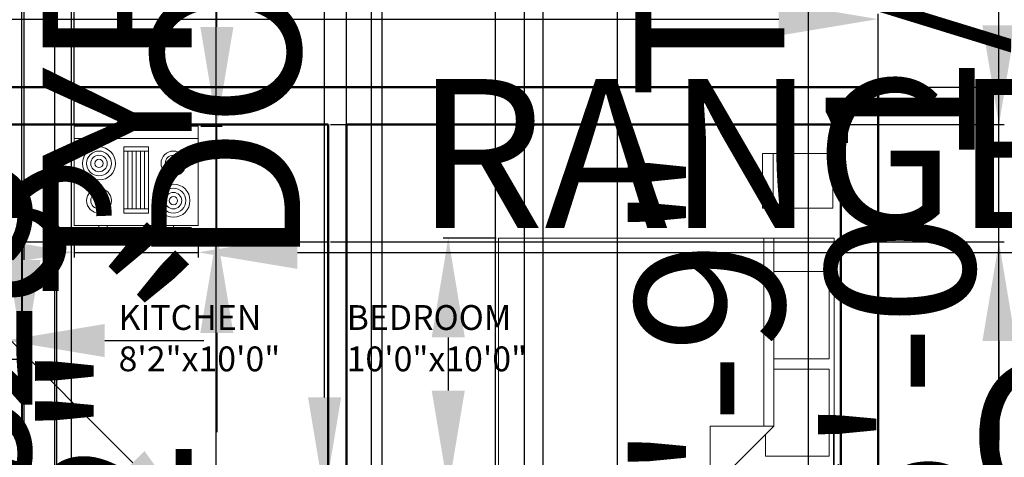
# Model space of a CAD drawing. Units: inches. Extents: x 1102 to 2414, y 295 to 1561.
# Tile 8 of 11: x 1610 to 1848, y 1027 to 1133. Entities that reach past the tile are written whole.
import ezdxf

# ---------------------------------------------------------------- set-up
doc = ezdxf.new("R2010")
doc.units = ezdxf.units.IN
for name, color, linetype, lineweight in [('A-ANNO-DIMS', 2, 'Continuous', 18), ('A-AREA-IDEN', 7, 'Continuous', 25), ('A-EQPM', 9, 'Continuous', 18), ('A-FLOR-CASE', 8, 'Continuous', 25), ('A-FURN', 8, 'Continuous', 18), ('A-WALL', 7, 'Continuous', 50)]:
    doc.layers.add(name, color=color, linetype=linetype, lineweight=lineweight)
doc.styles.get("Standard").update_dxf_attribs({"font": 'arial.ttf'})
doc.dimstyles.new('ISO-25', dxfattribs={"dimtxt": 36, "dimasz": 24, "dimexe": 1.25, "dimexo": 0.625, "dimtad": 1, "dimlunit": 4, "dimtxsty": 'Standard', "dimcen": 2.5, "dimadec": 0, "dimazin": 0, "dimtfac": 1, "dimtmove": 0, "dimatfit": 3, "dimfxl": 1, "dimarcsym": 0})

# ---------------------------------------------------------------- blocks, each defined once
blk = doc.blocks.new('*D1')
at = {"layer": 'A-ANNO-DIMS', "color": 0, "lineweight": -2, "transparency": 16777216}
for p, q in [((1577.54, 1117.38), (1577.54, 1134.48)), ((1817.54, 1117.38), (1817.54, 1134.48)), ((1601.54, 1133.23), (1793.54, 1133.23))]:
    blk.add_line(p, q, dxfattribs=at)
at = {"layer": 'A-ANNO-DIMS', "color": 0, "transparency": 16777216}
for points in [[(1601.54, 1137.23), (1601.54, 1129.23), (1577.54, 1133.23)], [(1793.54, 1137.23), (1793.54, 1129.23), (1817.54, 1133.23)]]:
    blk.add_solid(points, dxfattribs=at)
at = {"layer": 'Defpoints', "color": 0, "transparency": 16777216}
for p in [(1817.54, 1133.23), (1577.54, 1116.76), (1817.54, 1116.76)]:
    blk.add_point(p, dxfattribs=at)
at = {"layer": 'A-ANNO-DIMS', "color": 0, "transparency": 16777216, "insert": (1697.54, 1152.24), "char_height": 36, "attachment_point": 5}
blk.add_mtext("20'", dxfattribs=at)
blk = doc.blocks.new('*D3')
at = {"layer": 'A-ANNO-DIMS', "color": 0, "lineweight": -2, "transparency": 16777216}
for p, q in [((1818.17, 1116.76), (1895.42, 1116.76)), ((1894.17, 1092.76), (1894.17, 660.76)), ((1818.17, 636.76), (1895.42, 636.76))]:
    blk.add_line(p, q, dxfattribs=at)
at = {"layer": 'A-ANNO-DIMS', "color": 0, "transparency": 16777216}
for points in [[(1890.17, 1092.76), (1898.17, 1092.76), (1894.17, 1116.76)], [(1890.17, 660.76), (1898.17, 660.76), (1894.17, 636.76)]]:
    blk.add_solid(points, dxfattribs=at)
at = {"layer": 'Defpoints', "color": 0, "transparency": 16777216}
for p in [(1817.54, 1116.76), (1817.54, 636.76), (1894.17, 636.76)]:
    blk.add_point(p, dxfattribs=at)
at = {"layer": 'A-ANNO-DIMS', "color": 0, "transparency": 16777216, "insert": (1875.16, 876.76), "char_height": 36, "attachment_point": 5, "rotation": 90}
blk.add_mtext("40'", dxfattribs=at)
blk = doc.blocks.new('Range-Oven - 30 in top')
for p, q in [((0, -3), (30, -3)), ((12, -6), (18, -6)), ((13, -20), (13, -6)), ((14, -6), (14, -20)), ((15, -20), (15, -6)), ((16, -6), (16, -20)), ((17, -20), (17, -6)), ((18, -20), (12, -20)), ((6, -24), (6, -25)), ((8, -25), (8, -24)), ((22, -25), (22, -24)), ((24, -24), (24, -25))]:
    blk.add_line(p, q)
for points in [[(0, -24), (0, 0), (30, 0), (30, -24)], [(12, -21), (12, -5), (18, -5), (18, -21)], [(2, -26), (2, -25), (28, -25), (28, -26)]]:
    blk.add_lwpolyline(points, close=True)
for centre, radius in [((6, -9), 4), ((6, -9), 3), ((6, -9), 2), ((24, -9), 3), ((24, -9), 2), ((6, -9), 1), ((24, -9), 1), ((24, -18), 4), ((6, -18), 3), ((6, -18), 2), ((24, -18), 3), ((24, -18), 2), ((6, -18), 1), ((24, -18), 1)]:
    blk.add_circle(centre, radius)
blk = doc.blocks.new('Bed - Queen')
for p, q in [((0, -80.00003), (0, 0)), ((0, 0), (59.99999, 0)), ((59.99999, 0), (59.99999, -80.00003)), ((7.99999, -1.2), (28.79998, -1.2)), ((7.99999, -14.4), (7.99999, -1.2)), ((28.79998, -1.2), (28.79998, -14.4)), ((31.19999, -1.2), (51.99999, -1.2)), ((31.19999, -14.4), (31.19999, -1.2)), ((51.99999, -1.2), (51.99999, -16.4)), ((0, -14.4), (44.8, -14.4)), ((59.99999, -29.6), (44.8, -14.4)), ((44.8, -14.4), (44.8, -29.6)), ((51.99999, -16.4), (46.79936, -16.4)), ((44.8, -16.8), (0, -16.8)), ((44.8, -29.6), (59.99999, -29.6)), ((59.99999, -80.00003), (0, -80.00003))]:
    blk.add_line(p, q)
blk = doc.blocks.new('TABLE-BEDSIDE')
for p, q in [((16.99, 13.29), (0, 13.29)), ((0, 13.29), (0, 0)), ((2.56, 0), (2.56, 13.29)), ((16.99, 0), (16.99, 13.29)), ((0, 0), (16.99, 0))]:
    blk.add_line(p, q)
blk = doc.blocks.new('*D23')
at = {"layer": 'A-ANNO-DIMS', "color": 0, "lineweight": -2, "transparency": 16777216}
for p, q in [((1725.8, 1018.76), (1725.8, 1005.96)), ((1806.97, 1018.76), (1806.97, 1005.96)), ((1749.8, 1007.21), (1782.97, 1007.21)), ((1806.97, 1007.21), (2238.05, 1007.21))]:
    blk.add_line(p, q, dxfattribs=at)
at = {"layer": 'A-ANNO-DIMS', "color": 0, "transparency": 16777216}
for points in [[(1749.8, 1011.21), (1749.8, 1003.21), (1725.8, 1007.21)], [(1782.97, 1011.21), (1782.97, 1003.21), (1806.97, 1007.21)]]:
    blk.add_solid(points, dxfattribs=at)
at = {"layer": 'Defpoints', "color": 0, "transparency": 16777216}
for p in [(1725.8, 1019.39), (1806.97, 1019.39), (1806.97, 1007.21)]:
    blk.add_point(p, dxfattribs=at)
at = {"layer": 'A-ANNO-DIMS', "color": 0, "transparency": 16777216, "insert": (2034.51, 1027.55), "char_height": 36, "attachment_point": 5}
blk.add_mtext('QUEEN BED 6\'-9"', dxfattribs=at)
blk = doc.blocks.new('*D24')
at = {"layer": 'A-ANNO-DIMS', "color": 0, "lineweight": -2, "transparency": 16777216}
for p, q in [((1725.17, 1080.27), (1712.37, 1080.27)), ((1713.62, 1056.27), (1713.62, 1043.39)), ((1725.17, 1019.39), (1712.37, 1019.39)), ((1713.62, 1019.39), (1713.62, 898.44))]:
    blk.add_line(p, q, dxfattribs=at)
at = {"layer": 'A-ANNO-DIMS', "color": 0, "transparency": 16777216}
for points in [[(1709.62, 1056.27), (1717.62, 1056.27), (1713.62, 1080.27)], [(1709.62, 1043.39), (1717.62, 1043.39), (1713.62, 1019.39)]]:
    blk.add_solid(points, dxfattribs=at)
at = {"layer": 'Defpoints', "color": 0, "transparency": 16777216}
for p in [(1725.8, 1080.27), (1713.62, 1019.39), (1725.8, 1019.39)]:
    blk.add_point(p, dxfattribs=at)
at = {"layer": 'A-ANNO-DIMS', "color": 0, "transparency": 16777216, "insert": (1694.62, 946.91), "char_height": 36, "attachment_point": 5, "rotation": 90}
blk.add_mtext('5\'-1"', dxfattribs=at)
blk = doc.blocks.new('*D25')
at = {"layer": 'A-ANNO-DIMS', "color": 0, "lineweight": -2, "transparency": 16777216}
for p, q in [((1800.76, 877.69), (1800.76, 1221.61)), ((1796.43, 853.69), (1802.01, 853.69)), ((1800.76, 820.65), (1800.76, 853.69)), ((1796.43, 820.65), (1802.01, 820.65)), ((1800.76, 796.65), (1800.76, 772.65))]:
    blk.add_line(p, q, dxfattribs=at)
at = {"layer": 'A-ANNO-DIMS', "color": 0, "transparency": 16777216}
for points in [[(1796.76, 877.69), (1804.76, 877.69), (1800.76, 853.69)], [(1796.76, 796.65), (1804.76, 796.65), (1800.76, 820.65)]]:
    blk.add_solid(points, dxfattribs=at)
at = {"layer": 'Defpoints', "color": 0, "transparency": 16777216}
for p in [(1795.81, 853.69), (1800.76, 853.69), (1795.81, 820.65)]:
    blk.add_point(p, dxfattribs=at)
at = {"layer": 'A-ANNO-DIMS', "color": 0, "transparency": 16777216, "insert": (1781.53, 1061.65), "char_height": 36, "attachment_point": 5, "rotation": 90}
blk.add_mtext('WC 2\'-9" TYP.', dxfattribs=at)
blk = doc.blocks.new('*D27')
at = {"layer": 'A-ANNO-DIMS', "color": 0, "lineweight": -2, "transparency": 16777216}
for p, q in [((1683.72, 1041.76), (1683.72, 1561.36)), ((1679.17, 1017.76), (1684.97, 1017.76)), ((1683.72, 983.26), (1683.72, 1017.76)), ((1679.17, 983.26), (1684.97, 983.26)), ((1683.72, 959.26), (1683.72, 935.26))]:
    blk.add_line(p, q, dxfattribs=at)
at = {"layer": 'A-ANNO-DIMS', "color": 0, "transparency": 16777216}
for points in [[(1679.72, 1041.76), (1687.72, 1041.76), (1683.72, 1017.76)], [(1679.72, 959.26), (1687.72, 959.26), (1683.72, 983.26)]]:
    blk.add_solid(points, dxfattribs=at)
at = {"layer": 'Defpoints', "color": 0, "transparency": 16777216}
for p in [(1678.54, 1017.76), (1683.72, 1017.76), (1678.54, 983.26)]:
    blk.add_point(p, dxfattribs=at)
at = {"layer": 'A-ANNO-DIMS', "color": 0, "transparency": 16777216, "insert": (1664.47, 1313.56), "char_height": 36, "attachment_point": 5, "rotation": 90}
blk.add_mtext('DOOR 2\'-10 1/2" TYP.', dxfattribs=at)
blk = doc.blocks.new('*D28')
at = {"layer": 'A-ANNO-DIMS', "color": 0, "lineweight": -2, "transparency": 16777216}
for p, q in [((1645.54, 982.63), (1645.54, 976.83)), ((1678.54, 982.63), (1678.54, 976.83)), ((1621.54, 978.08), (1597.54, 978.08)), ((1645.54, 978.08), (1678.54, 978.08)), ((1702.54, 978.08), (1947.85, 978.08))]:
    blk.add_line(p, q, dxfattribs=at)
at = {"layer": 'A-ANNO-DIMS', "color": 0, "transparency": 16777216}
for points in [[(1621.54, 982.08), (1621.54, 974.08), (1645.54, 978.08)], [(1702.54, 982.08), (1702.54, 974.08), (1678.54, 978.08)]]:
    blk.add_solid(points, dxfattribs=at)
at = {"layer": 'Defpoints', "color": 0, "transparency": 16777216}
for p in [(1645.54, 983.26), (1678.54, 983.26), (1678.54, 978.08)]:
    blk.add_point(p, dxfattribs=at)
at = {"layer": 'A-ANNO-DIMS', "color": 0, "transparency": 16777216, "insert": (1837.19, 997.09), "char_height": 36, "attachment_point": 5}
blk.add_mtext('2\'-9" TYP.', dxfattribs=at)
blk = doc.blocks.new('*D29')
at = {"layer": 'A-ANNO-DIMS', "color": 0, "lineweight": -2, "transparency": 16777216}
for p, q in [((1806.82, 1011.76), (1806.82, 1035.76)), ((1803.17, 987.76), (1808.07, 987.76)), ((1806.82, 987.76), (1806.82, 959.26)), ((1803.17, 959.26), (1808.07, 959.26)), ((1806.82, 935.26), (1806.82, 295.33))]:
    blk.add_line(p, q, dxfattribs=at)
at = {"layer": 'A-ANNO-DIMS', "color": 0, "transparency": 16777216}
for points in [[(1802.82, 1011.76), (1810.82, 1011.76), (1806.82, 987.76)], [(1802.82, 935.26), (1810.82, 935.26), (1806.82, 959.26)]]:
    blk.add_solid(points, dxfattribs=at)
at = {"layer": 'Defpoints', "color": 0, "transparency": 16777216}
for p in [(1802.54, 987.76), (1802.54, 959.26), (1806.82, 959.26)]:
    blk.add_point(p, dxfattribs=at)
at = {"layer": 'A-ANNO-DIMS', "color": 0, "transparency": 16777216, "insert": (1787.57, 603.3), "char_height": 36, "attachment_point": 5, "rotation": 90}
blk.add_mtext('BATH DOOR 2\'-4 1/2" TYP.', dxfattribs=at)
blk = doc.blocks.new('*D30')
at = {"layer": 'A-ANNO-DIMS', "color": 0, "lineweight": -2, "transparency": 16777216}
for p, q in [((1775.54, 988.38), (1775.54, 993.28)), ((1802.54, 988.38), (1802.54, 993.28)), ((1751.54, 992.03), (1727.54, 992.03)), ((1775.54, 992.03), (1802.54, 992.03)), ((1826.54, 992.03), (2071.85, 992.03))]:
    blk.add_line(p, q, dxfattribs=at)
at = {"layer": 'A-ANNO-DIMS', "color": 0, "transparency": 16777216}
for points in [[(1751.54, 996.03), (1751.54, 988.03), (1775.54, 992.03)], [(1826.54, 996.03), (1826.54, 988.03), (1802.54, 992.03)]]:
    blk.add_solid(points, dxfattribs=at)
at = {"layer": 'Defpoints', "color": 0, "transparency": 16777216}
for p in [(1802.54, 992.03), (1775.54, 987.76), (1802.54, 987.76)]:
    blk.add_point(p, dxfattribs=at)
at = {"layer": 'A-ANNO-DIMS', "color": 0, "transparency": 16777216, "insert": (1961.19, 1011.05), "char_height": 36, "attachment_point": 5}
blk.add_mtext('2\'-3" TYP.', dxfattribs=at)
blk = doc.blocks.new('*D32')
at = {"layer": 'A-ANNO-DIMS', "color": 0, "lineweight": -2, "transparency": 16777216}
for p, q in [((1657.46, 811.76), (1657.46, 1164.91)), ((1654.49, 787.76), (1658.71, 787.76)), ((1657.46, 765.26), (1657.46, 787.76)), ((1654.49, 765.26), (1658.71, 765.26)), ((1657.46, 741.26), (1657.46, 717.26))]:
    blk.add_line(p, q, dxfattribs=at)
at = {"layer": 'A-ANNO-DIMS', "color": 0, "transparency": 16777216}
for points in [[(1653.46, 811.76), (1661.46, 811.76), (1657.46, 787.76)], [(1653.46, 741.26), (1661.46, 741.26), (1657.46, 765.26)]]:
    blk.add_solid(points, dxfattribs=at)
at = {"layer": 'Defpoints', "color": 0, "transparency": 16777216}
for p in [(1653.86, 787.76), (1657.46, 787.76), (1653.86, 765.26)]:
    blk.add_point(p, dxfattribs=at)
at = {"layer": 'A-ANNO-DIMS', "color": 0, "transparency": 16777216, "insert": (1638.22, 1000.34), "char_height": 36, "attachment_point": 5, "rotation": 90}
blk.add_mtext('1\'-10 1/2" TYP.', dxfattribs=at)
blk = doc.blocks.new('*D33')
at = {"layer": 'A-ANNO-DIMS', "color": 0, "lineweight": -2, "transparency": 16777216}
for p, q in [((1623.16, 1080.7), (1623.16, 1075.57)), ((1653.16, 1080.7), (1653.16, 1075.57)), ((1599.16, 1076.82), (1575.16, 1076.82)), ((1623.16, 1076.82), (1653.16, 1076.82)), ((1677.16, 1076.82), (1989.06, 1076.82))]:
    blk.add_line(p, q, dxfattribs=at)
at = {"layer": 'A-ANNO-DIMS', "color": 0, "transparency": 16777216}
for points in [[(1599.16, 1080.82), (1599.16, 1072.82), (1623.16, 1076.82)], [(1677.16, 1080.82), (1677.16, 1072.82), (1653.16, 1076.82)]]:
    blk.add_solid(points, dxfattribs=at)
at = {"layer": 'Defpoints', "color": 0, "transparency": 16777216}
for p in [(1623.16, 1081.32), (1653.16, 1081.32), (1653.16, 1076.82)]:
    blk.add_point(p, dxfattribs=at)
at = {"layer": 'A-ANNO-DIMS', "color": 0, "transparency": 16777216, "insert": (1845.11, 1096.06), "char_height": 36, "attachment_point": 5}
blk.add_mtext('RANGE 2\'-6"', dxfattribs=at)
blk = doc.blocks.new('*D34')
at = {"layer": 'A-ANNO-DIMS', "color": 0, "lineweight": -2, "transparency": 16777216}
for p, q in [((1657.66, 1131.32), (1657.66, 1252.88)), ((1653.79, 1107.32), (1658.91, 1107.32)), ((1657.66, 1081.32), (1657.66, 1107.32)), ((1653.79, 1081.32), (1658.91, 1081.32)), ((1657.66, 1057.32), (1657.66, 1033.32))]:
    blk.add_line(p, q, dxfattribs=at)
at = {"layer": 'A-ANNO-DIMS', "color": 0, "transparency": 16777216}
for points in [[(1653.66, 1131.32), (1661.66, 1131.32), (1657.66, 1107.32)], [(1653.66, 1057.32), (1661.66, 1057.32), (1657.66, 1081.32)]]:
    blk.add_solid(points, dxfattribs=at)
at = {"layer": 'Defpoints', "color": 0, "transparency": 16777216}
for p in [(1653.16, 1107.32), (1657.66, 1107.32), (1653.16, 1081.32)]:
    blk.add_point(p, dxfattribs=at)
at = {"layer": 'A-ANNO-DIMS', "color": 0, "transparency": 16777216, "insert": (1638.96, 1204.1), "char_height": 36, "attachment_point": 5, "rotation": 90}
blk.add_mtext('2\'-2"', dxfattribs=at)
blk = doc.blocks.new('*D35')
at = {"layer": 'A-ANNO-DIMS', "color": 0, "lineweight": -2, "transparency": 16777216}
for p, q in [((1611.04, 1074.99), (1611.04, 1327.12)), ((1607.17, 1050.99), (1612.29, 1050.99)), ((1611.04, 1020.99), (1611.04, 1050.99)), ((1607.17, 1020.99), (1612.29, 1020.99)), ((1611.04, 996.99), (1611.04, 972.99))]:
    blk.add_line(p, q, dxfattribs=at)
at = {"layer": 'A-ANNO-DIMS', "color": 0, "transparency": 16777216}
for points in [[(1607.04, 1074.99), (1615.04, 1074.99), (1611.04, 1050.99)], [(1607.04, 996.99), (1615.04, 996.99), (1611.04, 1020.99)]]:
    blk.add_solid(points, dxfattribs=at)
at = {"layer": 'Defpoints', "color": 0, "transparency": 16777216}
for p in [(1606.54, 1050.99), (1611.04, 1050.99), (1606.54, 1020.99)]:
    blk.add_point(p, dxfattribs=at)
at = {"layer": 'A-ANNO-DIMS', "color": 0, "transparency": 16777216, "insert": (1591.81, 1213.06), "char_height": 36, "attachment_point": 5, "rotation": 90}
blk.add_mtext('SINK 2\'-6"', dxfattribs=at)
blk = doc.blocks.new('*D36')
at = {"layer": 'A-ANNO-DIMS', "color": 0, "lineweight": -2, "transparency": 16777216}
for p, q in [((1562.54, 1055.49), (1444.99, 1055.49)), ((1586.54, 1051.62), (1586.54, 1056.74)), ((1606.54, 1055.49), (1586.54, 1055.49)), ((1606.54, 1051.62), (1606.54, 1056.74)), ((1630.54, 1055.49), (1654.54, 1055.49))]:
    blk.add_line(p, q, dxfattribs=at)
at = {"layer": 'A-ANNO-DIMS', "color": 0, "transparency": 16777216}
for points in [[(1562.54, 1059.49), (1562.54, 1051.49), (1586.54, 1055.49)], [(1630.54, 1059.49), (1630.54, 1051.49), (1606.54, 1055.49)]]:
    blk.add_solid(points, dxfattribs=at)
at = {"layer": 'Defpoints', "color": 0, "transparency": 16777216}
for p in [(1586.54, 1055.49), (1586.54, 1050.99), (1606.54, 1050.99)]:
    blk.add_point(p, dxfattribs=at)
at = {"layer": 'A-ANNO-DIMS', "color": 0, "transparency": 16777216, "insert": (1491.76, 1074.5), "char_height": 36, "attachment_point": 5}
blk.add_mtext('1\'-8"', dxfattribs=at)
blk = doc.blocks.new('*D37')
at = {"layer": 'A-ANNO-DIMS', "color": 0, "lineweight": -2, "transparency": 16777216}
for p, q in [((1618.46, 855.15), (1618.46, 1126.82)), ((1612.94, 831.15), (1619.71, 831.15)), ((1618.46, 790.23), (1618.46, 831.15)), ((1612.94, 790.23), (1619.71, 790.23)), ((1618.46, 766.23), (1618.46, 742.23))]:
    blk.add_line(p, q, dxfattribs=at)
at = {"layer": 'A-ANNO-DIMS', "color": 0, "transparency": 16777216}
for points in [[(1614.46, 855.15), (1622.46, 855.15), (1618.46, 831.15)], [(1614.46, 766.23), (1622.46, 766.23), (1618.46, 790.23)]]:
    blk.add_solid(points, dxfattribs=at)
at = {"layer": 'Defpoints', "color": 0, "transparency": 16777216}
for p in [(1612.32, 831.15), (1618.46, 831.15), (1612.32, 790.23)]:
    blk.add_point(p, dxfattribs=at)
at = {"layer": 'A-ANNO-DIMS', "color": 0, "transparency": 16777216, "insert": (1599.19, 1002.98), "char_height": 36, "attachment_point": 5, "rotation": 90}
blk.add_mtext('SOFA 3\'-5"', dxfattribs=at)
blk = doc.blocks.new('*D40')
at = {"layer": 'A-ANNO-DIMS', "color": 0, "lineweight": -2, "transparency": 16777216}
for p, q in [((1618.98, 879.05), (1618.98, 1080.49)), ((1622.7, 855.05), (1617.73, 855.05)), ((1618.98, 837.36), (1618.98, 855.05)), ((1622.7, 837.36), (1617.73, 837.36)), ((1618.98, 813.36), (1618.98, 789.36))]:
    blk.add_line(p, q, dxfattribs=at)
at = {"layer": 'A-ANNO-DIMS', "color": 0, "transparency": 16777216}
for points in [[(1614.98, 879.05), (1622.98, 879.05), (1618.98, 855.05)], [(1614.98, 813.36), (1622.98, 813.36), (1618.98, 837.36)]]:
    blk.add_solid(points, dxfattribs=at)
at = {"layer": 'Defpoints', "color": 0, "transparency": 16777216}
for p in [(1618.98, 855.05), (1623.32, 855.05), (1623.32, 837.36)]:
    blk.add_point(p, dxfattribs=at)
at = {"layer": 'A-ANNO-DIMS', "color": 0, "transparency": 16777216, "insert": (1599.74, 991.77), "char_height": 36, "attachment_point": 5, "rotation": 90}
blk.add_mtext('1\'-5 1/2"', dxfattribs=at)
blk = doc.blocks.new('*D45')
at = {"layer": 'A-ANNO-DIMS', "color": 0, "lineweight": -2, "transparency": 16777216}
for p, q in [((1712.54, 1146.01), (1688.54, 1146.01)), ((1736.54, 770.38), (1736.54, 1147.26)), ((1736.54, 1146.01), (1754.54, 1146.01)), ((1754.54, 770.38), (1754.54, 1147.26)), ((1778.54, 1146.01), (1896.1, 1146.01))]:
    blk.add_line(p, q, dxfattribs=at)
at = {"layer": 'A-ANNO-DIMS', "color": 0, "transparency": 16777216}
for points in [[(1712.54, 1150.01), (1712.54, 1142.01), (1736.54, 1146.01)], [(1778.54, 1150.01), (1778.54, 1142.01), (1754.54, 1146.01)]]:
    blk.add_solid(points, dxfattribs=at)
at = {"layer": 'Defpoints', "color": 0, "transparency": 16777216}
for p in [(1754.54, 1146.01), (1736.54, 769.76), (1754.54, 769.76)]:
    blk.add_point(p, dxfattribs=at)
at = {"layer": 'A-ANNO-DIMS', "color": 0, "transparency": 16777216, "insert": (1849.32, 1165.02), "char_height": 36, "attachment_point": 5}
blk.add_mtext('1\'-6"', dxfattribs=at)
blk = doc.blocks.new('*D48')
at = {"layer": 'A-ANNO-DIMS', "color": 0, "lineweight": -2, "transparency": 16777216}
for p, q in [((1665.04, 1146.01), (1641.04, 1146.01)), ((1689.04, 854.38), (1689.04, 1147.26)), ((1689.04, 1146.01), (1732.04, 1146.01)), ((1732.04, 858.88), (1732.04, 1147.26)), ((1756.04, 1146.01), (1876.97, 1146.01))]:
    blk.add_line(p, q, dxfattribs=at)
at = {"layer": 'A-ANNO-DIMS', "color": 0, "transparency": 16777216}
for points in [[(1665.04, 1150.01), (1665.04, 1142.01), (1689.04, 1146.01)], [(1756.04, 1150.01), (1756.04, 1142.01), (1732.04, 1146.01)]]:
    blk.add_solid(points, dxfattribs=at)
at = {"layer": 'Defpoints', "color": 0, "transparency": 16777216}
for p in [(1732.04, 1146.01), (1732.04, 858.26), (1689.04, 853.76)]:
    blk.add_point(p, dxfattribs=at)
at = {"layer": 'A-ANNO-DIMS', "color": 0, "transparency": 16777216, "insert": (1828.51, 1165.03), "char_height": 36, "attachment_point": 5}
blk.add_mtext('3\'-7"', dxfattribs=at)
blk = doc.blocks.new('*D49')
at = {"layer": 'A-ANNO-DIMS', "color": 0, "lineweight": -2, "transparency": 16777216}
for p, q in [((1846.79, 983.26), (1846.79, 1188.29)), ((1809.17, 983.26), (1848.04, 983.26)), ((1846.79, 934.76), (1846.79, 959.26)), ((1809.17, 910.76), (1848.04, 910.76))]:
    blk.add_line(p, q, dxfattribs=at)
at = {"layer": 'A-ANNO-DIMS', "color": 0, "transparency": 16777216}
for points in [[(1842.79, 959.26), (1850.79, 959.26), (1846.79, 983.26)], [(1842.79, 934.76), (1850.79, 934.76), (1846.79, 910.76)]]:
    blk.add_solid(points, dxfattribs=at)
at = {"layer": 'Defpoints', "color": 0, "transparency": 16777216}
for p in [(1808.54, 983.26), (1846.79, 983.26), (1808.54, 910.76)]:
    blk.add_point(p, dxfattribs=at)
at = {"layer": 'A-ANNO-DIMS', "color": 0, "transparency": 16777216, "insert": (1827.56, 1097.77), "char_height": 36, "attachment_point": 5, "rotation": 90}
blk.add_mtext('6\'-0 1/2"', dxfattribs=at)
blk = doc.blocks.new('*D51')
at = {"layer": 'A-ANNO-DIMS', "color": 0, "lineweight": -2, "transparency": 16777216}
for p, q in [((1665.04, 1146.01), (1641.04, 1146.01)), ((1689.04, 988.38), (1689.04, 1147.26)), ((1689.04, 1146.01), (1695.04, 1146.01)), ((1695.04, 988.38), (1695.04, 1147.26)), ((1719.04, 1146.01), (1839.99, 1146.01))]:
    blk.add_line(p, q, dxfattribs=at)
at = {"layer": 'A-ANNO-DIMS', "color": 0, "transparency": 16777216}
for points in [[(1665.04, 1150.01), (1665.04, 1142.01), (1689.04, 1146.01)], [(1719.04, 1150.01), (1719.04, 1142.01), (1695.04, 1146.01)]]:
    blk.add_solid(points, dxfattribs=at)
at = {"layer": 'Defpoints', "color": 0, "transparency": 16777216}
for p in [(1695.04, 1146.01), (1689.04, 987.76), (1695.04, 987.76)]:
    blk.add_point(p, dxfattribs=at)
at = {"layer": 'A-ANNO-DIMS', "color": 0, "transparency": 16777216, "insert": (1791.52, 1165.02), "char_height": 36, "attachment_point": 5}
blk.add_mtext('0\'-6"', dxfattribs=at)
blk = doc.blocks.new('*D52')
at = {"layer": 'A-ANNO-DIMS', "color": 0, "lineweight": -2, "transparency": 16777216}
for p, q in [((1778.54, 1017.01), (1754.54, 1017.01)), ((1802.54, 988.38), (1802.54, 1018.26)), ((1802.54, 1017.01), (1808.54, 1017.01)), ((1808.54, 988.38), (1808.54, 1018.26)), ((1832.54, 1017.01), (1953.49, 1017.01))]:
    blk.add_line(p, q, dxfattribs=at)
at = {"layer": 'A-ANNO-DIMS', "color": 0, "transparency": 16777216}
for points in [[(1778.54, 1021.01), (1778.54, 1013.01), (1802.54, 1017.01)], [(1832.54, 1021.01), (1832.54, 1013.01), (1808.54, 1017.01)]]:
    blk.add_solid(points, dxfattribs=at)
at = {"layer": 'Defpoints', "color": 0, "transparency": 16777216}
for p in [(1808.54, 1017.01), (1802.54, 987.76), (1808.54, 987.76)]:
    blk.add_point(p, dxfattribs=at)
at = {"layer": 'A-ANNO-DIMS', "color": 0, "transparency": 16777216, "insert": (1905.02, 1036.02), "char_height": 36, "attachment_point": 5}
blk.add_mtext('0\'-6"', dxfattribs=at)
blk = doc.blocks.new('*D53')
at = {"layer": 'A-ANNO-DIMS', "color": 0, "lineweight": -2, "transparency": 16777216}
for p, q in [((1562.54, 1146.01), (1538.54, 1146.01)), ((1586.54, 988.38), (1586.54, 1147.26)), ((1586.54, 1146.01), (1610.54, 1146.01)), ((1610.54, 988.38), (1610.54, 1147.26)), ((1634.54, 1146.01), (1756.11, 1146.01))]:
    blk.add_line(p, q, dxfattribs=at)
at = {"layer": 'A-ANNO-DIMS', "color": 0, "transparency": 16777216}
for points in [[(1562.54, 1150.01), (1562.54, 1142.01), (1586.54, 1146.01)], [(1634.54, 1150.01), (1634.54, 1142.01), (1610.54, 1146.01)]]:
    blk.add_solid(points, dxfattribs=at)
at = {"layer": 'Defpoints', "color": 0, "transparency": 16777216}
for p in [(1610.54, 1146.01), (1586.54, 987.76), (1610.54, 987.76)]:
    blk.add_point(p, dxfattribs=at)
at = {"layer": 'A-ANNO-DIMS', "color": 0, "transparency": 16777216, "insert": (1707.32, 1165.02), "char_height": 36, "attachment_point": 5}
blk.add_mtext('2\'-0"', dxfattribs=at)
blk = doc.blocks.new('*D54')
at = {"layer": 'A-ANNO-DIMS', "color": 0, "lineweight": -2, "transparency": 16777216}
for p, q in [((1846.79, 1131.76), (1846.79, 1337.21)), ((1685.17, 1107.76), (1848.04, 1107.76)), ((1846.79, 1079.39), (1846.79, 1107.76)), ((1685.17, 1079.39), (1848.04, 1079.39)), ((1846.79, 1055.39), (1846.79, 1031.39))]:
    blk.add_line(p, q, dxfattribs=at)
at = {"layer": 'A-ANNO-DIMS', "color": 0, "transparency": 16777216}
for points in [[(1842.79, 1131.76), (1850.79, 1131.76), (1846.79, 1107.76)], [(1842.79, 1055.39), (1850.79, 1055.39), (1846.79, 1079.39)]]:
    blk.add_solid(points, dxfattribs=at)
at = {"layer": 'Defpoints', "color": 0, "transparency": 16777216}
for p in [(1684.54, 1107.76), (1846.79, 1107.76), (1684.54, 1079.39)]:
    blk.add_point(p, dxfattribs=at)
at = {"layer": 'A-ANNO-DIMS', "color": 0, "transparency": 16777216, "insert": (1827.56, 1246.48), "char_height": 36, "attachment_point": 5, "rotation": 90}
blk.add_mtext('2\'-4 1/2"', dxfattribs=at)
blk = doc.blocks.new('*D55')
at = {"layer": 'A-ANNO-DIMS', "color": 0, "lineweight": -2, "transparency": 16777216}
for p, q in [((1562.54, 1146.01), (1538.54, 1146.01)), ((1586.54, 722.38), (1586.54, 1147.26)), ((1586.54, 1146.01), (1622.54, 1146.01)), ((1622.54, 722.38), (1622.54, 1147.26)), ((1646.54, 1146.01), (1767.47, 1146.01))]:
    blk.add_line(p, q, dxfattribs=at)
at = {"layer": 'A-ANNO-DIMS', "color": 0, "transparency": 16777216}
for points in [[(1562.54, 1150.01), (1562.54, 1142.01), (1586.54, 1146.01)], [(1646.54, 1150.01), (1646.54, 1142.01), (1622.54, 1146.01)]]:
    blk.add_solid(points, dxfattribs=at)
at = {"layer": 'Defpoints', "color": 0, "transparency": 16777216}
for p in [(1622.54, 1146.01), (1586.54, 721.76), (1622.54, 721.76)]:
    blk.add_point(p, dxfattribs=at)
at = {"layer": 'A-ANNO-DIMS', "color": 0, "transparency": 16777216, "insert": (1719.01, 1165.03), "char_height": 36, "attachment_point": 5}
blk.add_mtext('3\'-0"', dxfattribs=at)
blk = doc.blocks.new('*D59')
at = {"layer": 'A-ANNO-DIMS', "color": 0, "lineweight": -2, "transparency": 16777216}
for p, q in [((1548.29, 962.66), (1548.29, 1112.19)), ((1612.15, 938.66), (1547.04, 938.66)), ((1548.29, 903.8), (1548.29, 938.66)), ((1612.15, 903.8), (1547.04, 903.8)), ((1548.29, 879.8), (1548.29, 855.8))]:
    blk.add_line(p, q, dxfattribs=at)
at = {"layer": 'A-ANNO-DIMS', "color": 0, "transparency": 16777216}
for points in [[(1544.29, 962.66), (1552.29, 962.66), (1548.29, 938.66)], [(1544.29, 879.8), (1552.29, 879.8), (1548.29, 903.8)]]:
    blk.add_solid(points, dxfattribs=at)
at = {"layer": 'Defpoints', "color": 0, "transparency": 16777216}
for p in [(1548.29, 938.66), (1612.78, 938.66), (1612.78, 903.8)]:
    blk.add_point(p, dxfattribs=at)
at = {"layer": 'A-ANNO-DIMS', "color": 0, "transparency": 16777216, "insert": (1529.6, 1049.43), "char_height": 36, "attachment_point": 5, "rotation": 90}
blk.add_mtext('2\'-11"', dxfattribs=at)
blk = doc.blocks.new('*D60')
at = {"layer": 'A-ANNO-DIMS', "color": 0, "lineweight": -2, "transparency": 16777216}
for p, q in [((1562.54, 1146.01), (1538.54, 1146.01)), ((1586.54, 1108.38), (1586.54, 1147.26)), ((1586.54, 1146.01), (1623.16, 1146.01)), ((1623.16, 1107.95), (1623.16, 1147.26)), ((1647.16, 1146.01), (1851.97, 1146.01))]:
    blk.add_line(p, q, dxfattribs=at)
at = {"layer": 'A-ANNO-DIMS', "color": 0, "transparency": 16777216}
for points in [[(1562.54, 1150.01), (1562.54, 1142.01), (1586.54, 1146.01)], [(1647.16, 1150.01), (1647.16, 1142.01), (1623.16, 1146.01)]]:
    blk.add_solid(points, dxfattribs=at)
at = {"layer": 'Defpoints', "color": 0, "transparency": 16777216}
for p in [(1623.16, 1146.01), (1586.54, 1107.76), (1623.16, 1107.32)]:
    blk.add_point(p, dxfattribs=at)
at = {"layer": 'A-ANNO-DIMS', "color": 0, "transparency": 16777216, "insert": (1761.57, 1165.26), "char_height": 36, "attachment_point": 5}
blk.add_mtext('3\'-0 1/2"', dxfattribs=at)
blk = doc.blocks.new('*D65')
at = {"layer": 'A-ANNO-DIMS', "color": 0, "lineweight": -2, "transparency": 16777216}
for p, q in [((1673.64, 1146.01), (1649.64, 1146.01)), ((1697.64, 770.38), (1697.64, 1147.26)), ((1697.64, 1146.01), (1725.04, 1146.01)), ((1725.04, 770.38), (1725.04, 1147.26)), ((1749.04, 1146.01), (1954.49, 1146.01))]:
    blk.add_line(p, q, dxfattribs=at)
at = {"layer": 'A-ANNO-DIMS', "color": 0, "transparency": 16777216}
for points in [[(1673.64, 1150.01), (1673.64, 1142.01), (1697.64, 1146.01)], [(1749.04, 1150.01), (1749.04, 1142.01), (1725.04, 1146.01)]]:
    blk.add_solid(points, dxfattribs=at)
at = {"layer": 'Defpoints', "color": 0, "transparency": 16777216}
for p in [(1725.04, 1146.01), (1697.64, 769.76), (1725.04, 769.76)]:
    blk.add_point(p, dxfattribs=at)
at = {"layer": 'A-ANNO-DIMS', "color": 0, "transparency": 16777216, "insert": (1863.77, 1165.26), "char_height": 36, "attachment_point": 5}
blk.add_mtext('2\'-3 1/2"', dxfattribs=at)
blk = doc.blocks.new('*D68')
at = {"layer": 'A-ANNO-DIMS', "color": 0, "lineweight": -2, "transparency": 16777216}
for p, q in [((1527.48, 1135.83), (1637.36, 1025.94)), ((1675.54, 987.76), (1654.33, 1008.97))]:
    blk.add_line(p, q, dxfattribs=at)
at = {"layer": 'A-ANNO-DIMS', "color": 0, "transparency": 16777216}
blk.add_solid([(1640.19, 1028.77), (1634.53, 1023.12), (1654.33, 1008.97)], dxfattribs=at)
at = {"layer": 'Defpoints', "color": 0, "transparency": 16777216}
for p in [(1654.33, 1008.97), (1675.54, 987.76)]:
    blk.add_point(p, dxfattribs=at)
at = {"layer": 'A-ANNO-DIMS', "color": 0, "transparency": 16777216, "insert": (1587.37, 1102.81), "char_height": 36, "attachment_point": 5, "rotation": 314.9996}
blk.add_mtext('R2\'-6"', dxfattribs=at)

msp = doc.modelspace()

# ---------------------------------------------------------------- linework, layer by layer
at = {"layer": 'A-FLOR-CASE'}
for q in [(1610.544, 987.76), (1684.544, 1079.395)]:
    msp.add_line((1610.544, 1079.395), q, dxfattribs=at)
at = {"layer": 'A-WALL'}
for p, q in [((1817.544, 1116.76), (1577.544, 1116.76)), ((1817.544, 636.76), (1817.544, 1116.76)), ((1684.544, 1107.76), (1586.544, 1107.76)), ((1684.544, 1107.76), (1684.544, 987.76)), ((1808.544, 1107.76), (1689.044, 1107.76)), ((1689.044, 1107.76), (1689.044, 987.76)), ((1808.544, 987.76), (1808.544, 1107.76))]:
    msp.add_line(p, q, dxfattribs=at)

# ---------------------------------------------------------------- block references
at = {"layer": 'A-EQPM'}
msp.add_blockref('Range-Oven - 30 in top', (1623.162, 1107.321), dxfattribs=at)
at = {"layer": 'A-FURN'}
msp.add_blockref('TABLE-BEDSIDE', (1789.608, 1087.467), dxfattribs=at)
at = {"layer": 'A-FURN', "xscale": 1.014688796722326, "yscale": 1.014688796722326, "zscale": 1.014688796722326, "rotation": 270}
msp.add_blockref('Bed - Queen', (1806.973, 1080.268), dxfattribs=at)

# ---------------------------------------------------------------- texts
at = {"layer": 'A-AREA-IDEN', "char_height": 6, "attachment_point": 1}
for s, insert in [('KITCHEN\\P8\'2"x10\'0"', (1633.895, 1064.066)), ('BEDROOM\\P10\'0"x10\'0"', (1689.044, 1064.066))]:
    msp.add_mtext_dynamic_manual_height_columns(s, width=50.64919, gutter_width=12.5, heights=[0], dxfattribs=dict(at, insert=insert))

# ---------------------------------------------------------------- dimensions: what is measured, and where the dimension line sits
at = {"layer": 'A-ANNO-DIMS'}
for base, p1, p2, angle, text, picture, middle in [((1683.719, 1017.76), (1678.544, 983.26), (1678.544, 1017.76), 90, 'DOOR <> TYP.', '*D27', (1664.468, 1313.559)), ((1611.044, 1050.991), (1606.544, 1020.991), (1606.544, 1050.991), 90, 'SINK <>', '*D35', (1591.805, 1213.055)), ((1800.764, 853.692), (1795.807, 820.646), (1795.807, 853.692), 90, 'WC <> TYP.', '*D25', (1781.525, 1061.653)), ((1657.464, 787.76), (1653.864, 765.26), (1653.864, 787.76), 90, '<> TYP.', '*D32', (1638.225, 1000.337)), ((1618.456, 831.145), (1612.319, 790.233), (1612.319, 831.145), 90, 'SOFA <>', '*D37', (1599.192, 1002.983)), ((1806.819, 959.26), (1802.544, 987.76), (1802.544, 959.26), 270, 'BATH DOOR <> TYP.', '*D29', (1787.568, 603.296))]:
    dim = msp.add_linear_dim(base=base, p1=p1, p2=p2, angle=angle, text=text, dimstyle='ISO-25', override={"dimdec": 1, "dimlfac": 1, "dimrnd": 0, "dimzin": 1, "dimdsep": 46, "dimlunit": 4, "dimfrac": 2}, dxfattribs=at)
    dim.commit()
    dim.dimension.update_dxf_attribs({"geometry": picture, "text_midpoint": middle})
for base, p1, p2, angle, picture, middle in [((1846.794, 1107.76), (1684.544, 1079.395), (1684.544, 1107.76), 90, '*D54', (1827.555, 1246.483)), ((1657.662, 1107.321), (1653.162, 1081.321), (1653.162, 1107.321), 90, '*D34', (1638.964, 1204.102)), ((1846.794, 983.26), (1808.544, 910.76), (1808.544, 983.26), 90, '*D49', (1827.555, 1097.774)), ((1548.294, 938.663), (1612.778, 903.803), (1612.778, 938.663), 90, '*D59', (1529.595, 1049.429)), ((1586.544, 1055.491), (1606.544, 1050.991), (1586.544, 1050.991), 180, '*D36', (1491.765, 1074.497)), ((1618.978, 855.046), (1623.32, 837.356), (1623.32, 855.046), 90, '*D40', (1599.739, 991.768)), ((1713.621, 1019.387), (1725.798, 1080.268), (1725.798, 1019.387), 270, '*D24', (1694.616, 946.913))]:
    dim = msp.add_linear_dim(base=base, p1=p1, p2=p2, angle=angle, dimstyle='ISO-25', override={"dimdec": 1, "dimlfac": 1, "dimrnd": 0, "dimzin": 1, "dimdsep": 46, "dimlunit": 4, "dimfrac": 2}, dxfattribs=at)
    dim.commit()
    dim.dimension.update_dxf_attribs({"geometry": picture, "text_midpoint": middle})
for base, p1, p2, override, picture, middle in [((1623.162, 1146.01), (1586.544, 1107.76), (1623.162, 1107.321), {"dimdec": 1, "dimlfac": 1, "dimrnd": 0, "dimzin": 1, "dimdsep": 46, "dimlunit": 4, "dimfrac": 2}, '*D60', (1761.566, 1165.261)), ((1725.044, 1146.01), (1697.644, 769.76), (1725.044, 769.76), {"dimdec": 1, "dimlfac": 1, "dimrnd": 0, "dimzin": 1, "dimdsep": 46, "dimlunit": 4, "dimfrac": 2}, '*D65', (1863.767, 1165.261)), ((1622.544, 1146.01), (1586.544, 721.76), (1622.544, 721.76), {"dimdec": 1, "dimlfac": 1, "dimrnd": 0, "dimzin": 1, "dimdsep": 46, "dimlunit": 4, "dimfrac": 2}, '*D55', (1719.005, 1165.028)), ((1610.544, 1146.01), (1586.544, 987.76), (1610.544, 987.76), {"dimdec": 1, "dimlfac": 1, "dimrnd": 0, "dimzin": 1, "dimdsep": 46, "dimlunit": 4, "dimfrac": 2}, '*D53', (1707.325, 1165.015)), ((1732.044, 1146.01), (1689.044, 853.76), (1732.044, 858.26), {"dimdec": 1, "dimlfac": 1, "dimrnd": 0, "dimzin": 1, "dimdsep": 46, "dimlunit": 4, "dimfrac": 2}, '*D48', (1828.505, 1165.028)), ((1695.044, 1146.01), (1689.044, 987.76), (1695.044, 987.76), {"dimdec": 1, "dimlfac": 1, "dimrnd": 0, "dimzin": 1, "dimdsep": 46, "dimlunit": 4, "dimfrac": 2}, '*D51', (1791.518, 1165.015)), ((1754.544, 1146.01), (1736.544, 769.76), (1754.544, 769.76), {"dimdec": 1, "dimlfac": 1, "dimrnd": 0, "dimzin": 1, "dimdsep": 46, "dimlunit": 4, "dimfrac": 2}, '*D45', (1849.323, 1165.015)), ((1817.544, 1133.235), (1577.544, 1116.76), (1817.544, 1116.76), {"dimclrd": 0, "dimclre": 0, "dimclrt": 0}, '*D1', (1697.544, 1152.24)), ((1808.544, 1017.01), (1802.544, 987.76), (1808.544, 987.76), {"dimdec": 1, "dimlfac": 1, "dimrnd": 0, "dimzin": 1, "dimdsep": 46, "dimlunit": 4, "dimfrac": 2}, '*D52', (1905.018, 1036.015))]:
    dim = msp.add_linear_dim(base=base, p1=p1, p2=p2, dimstyle='ISO-25', override=override, dxfattribs=at)
    dim.commit()
    dim.dimension.update_dxf_attribs({"geometry": picture, "text_midpoint": middle})
dim = msp.add_radius_dim(center=(1675.544, 987.76), mpoint=(1654.331, 1008.973), dimstyle='ISO-25', override={"dimdec": 1, "dimlfac": 1, "dimrnd": 0, "dimzin": 1, "dimdsep": 46, "dimlunit": 4, "dimfrac": 2}, dxfattribs=at)
dim.commit()
dim.dimension.update_dxf_attribs({"geometry": '*D68', "text_midpoint": (1587.373, 1102.811)})
for base, p1, p2, text, picture, middle in [((1653.162, 1076.821), (1623.162, 1081.321), (1653.162, 1081.321), 'RANGE <>', '*D33', (1845.112, 1096.06)), ((1806.973, 1007.211), (1725.798, 1019.387), (1806.973, 1019.387), 'QUEEN BED <>', '*D23', (2034.509, 1027.555)), ((1802.544, 992.035), (1775.544, 987.76), (1802.544, 987.76), '<> TYP.', '*D30', (1961.195, 1011.053)), ((1678.544, 978.085), (1645.544, 983.26), (1678.544, 983.26), '<> TYP.', '*D28', (1837.195, 997.09))]:
    dim = msp.add_linear_dim(base=base, p1=p1, p2=p2, text=text, dimstyle='ISO-25', override={"dimdec": 1, "dimlfac": 1, "dimrnd": 0, "dimzin": 1, "dimdsep": 46, "dimlunit": 4, "dimfrac": 2}, dxfattribs=at)
    dim.commit()
    dim.dimension.update_dxf_attribs({"geometry": picture, "text_midpoint": middle})
dim = msp.add_linear_dim(base=(1894.167, 636.76), p1=(1817.544, 1116.76), p2=(1817.544, 636.76), angle=90, dimstyle='ISO-25', override={"dimclrd": 0, "dimclre": 0, "dimclrt": 0}, dxfattribs=at)
dim.commit()
dim.dimension.update_dxf_attribs({"geometry": '*D3', "text_midpoint": (1894.167, 876.76), "dimtype": 160})

doc.saveas('drawing.dxf')
